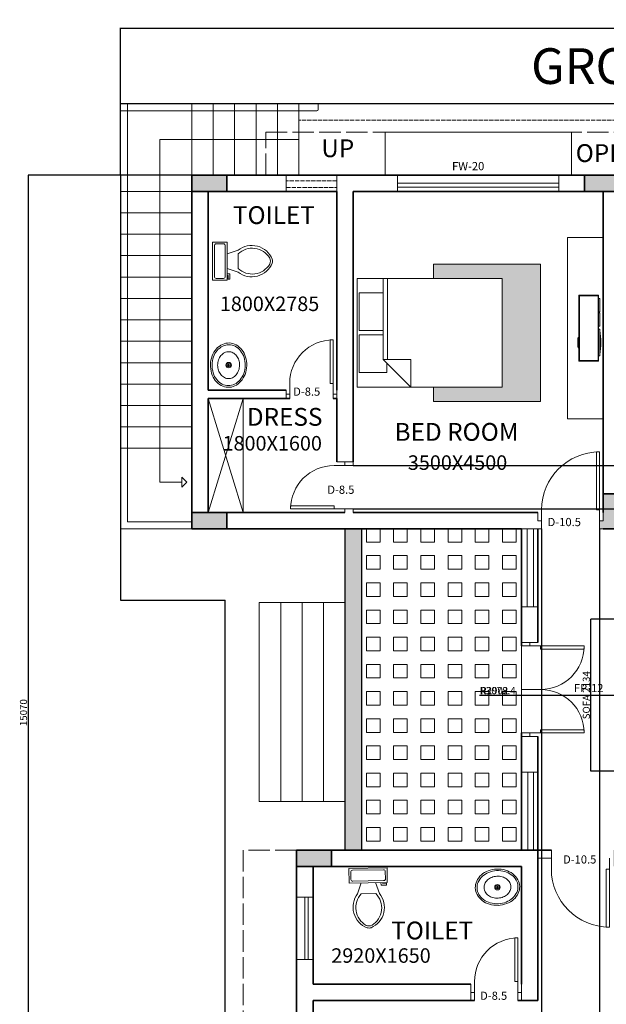
# Model space of a CAD drawing. Units: millimetres. Extents: x -17016 to 4866, y -18325 to 4338.
# Tile 2 of 5: x -17016 to -8803, y -9462 to 4338. Entities that reach past the tile are written whole.
import ezdxf

# ---------------------------------------------------------------- set-up
doc = ezdxf.new("R2010")
doc.units = ezdxf.units.MM
doc.header["$LTSCALE"] = 5
doc.linetypes.add('ACAD_ISO02W100', pattern=[15, 12, -3])
for name, color, linetype, lineweight in [('A-ANNO-DIMS', 2, 'Continuous', 18), ('A-ANNO-IDEN', 3, 'Continuous', 18), ('A-ANNO-SYMB', 7, 'Continuous', 18), ('A-ANNO-TEXT', 7, 'Continuous', 25), ('A-AREA-IDEN', 7, 'Continuous', 25), ('A-COLS', 7, 'Continuous', 35), ('A-COLS-PATT', 252, 'Continuous', 13), ('A-DOOR', 3, 'Continuous', 18), ('A-FLOR-CASE', 8, 'Continuous', 18), ('A-FLOR-FIXT', 9, 'Continuous', 18), ('A-FLOR-OTLN', 8, 'Continuous', 25), ('A-FLOR-PATT', 252, 'Continuous', 13), ('A-FLOR-STRS', 7, 'Continuous', 18), ('A-FURN', 8, 'Continuous', 18), ('A-GLAZ', 4, 'Continuous', 18), ('A-GLAZ-HIDN', 4, 'ACAD_ISO02W100', 18), ('A-ROOF', 8, 'Continuous', 18), ('A-ROOF-OVHD', 8, 'ACAD_ISO02W100', 13), ('A-WALL', 7, 'Continuous', 35)]:
    doc.layers.add(name, color=color, linetype=linetype, lineweight=lineweight)
doc.styles.get("Standard").update_dxf_attribs({"font": 'arial.ttf'})
doc.dimstyles.new('Copy of ISO-25', dxfattribs={"dimtxt": 100, "dimasz": 2.5, "dimexe": 1.25, "dimexo": 0.625, "dimtad": 1, "dimdec": 0, "dimtxsty": 'Standard', "dimcen": 2.5, "dimadec": 0, "dimazin": 0, "dimtfac": 1, "dimtdec": 0, "dimtmove": 0, "dimatfit": 3, "dimfxl": 1, "dimarcsym": 0})

# ---------------------------------------------------------------- blocks, each defined once
blk = doc.blocks.new('*U2')
for p, q in [((0, 0), (0, -6)), ((32, 0), (32, -6))]:
    blk.add_line(p, q)
blk.add_lwpolyline([(0, 0), (0, 32), (1.75, 32), (1.75, 0)], close=True)
blk.add_arc((0, 0), 32, 0, 90)
blk = doc.blocks.new('*U3')
for p, q in [((0, 0), (0, -6)), ((24, 0), (24, -6))]:
    blk.add_line(p, q)
blk.add_lwpolyline([(0, 0), (0, 24), (1.75, 24), (1.75, 0)], close=True)
blk.add_arc((0, 0), 24, 0, 90)
blk = doc.blocks.new('Bed - Queen')
for p, q in [((0, -80.00003), (0, 0)), ((0, 0), (59.99999, 0)), ((59.99999, 0), (59.99999, -80.00003)), ((7.99999, -1.2), (28.79998, -1.2)), ((7.99999, -14.4), (7.99999, -1.2)), ((28.79998, -1.2), (28.79998, -14.4)), ((31.19999, -1.2), (51.99999, -1.2)), ((31.19999, -14.4), (31.19999, -1.2)), ((51.99999, -1.2), (51.99999, -16.4)), ((0, -14.4), (44.8, -14.4)), ((59.99999, -29.6), (44.8, -14.4)), ((44.8, -14.4), (44.8, -29.6)), ((44.8, -16.8), (0, -16.8)), ((51.99999, -16.4), (46.79936, -16.4)), ((44.8, -29.6), (59.99999, -29.6)), ((59.99999, -80.00003), (0, -80.00003))]:
    blk.add_line(p, q)
blk = doc.blocks.new('Entertainment Center')
for p, q in [((-4, 0), (-5, -1)), ((4, 0), (-4, 0)), ((5, -1), (4, 0)), ((-17, -19), (-17, -1)), ((-17, -1), (43, -1)), ((-16.5, -18.5), (-16.5, -1.5)), ((-16.5, -1.5), (42.5, -1.5)), ((42.5, -1.5), (42.5, -18.5)), ((43, -1), (43, -19)), ((43, -19), (-17, -19)), ((42.5, -18.5), (-16.5, -18.5)), ((-12, -20), (-12, -19)), ((12, -20), (-12, -20)), ((12, -19), (12, -20)), ((15, -20), (15, -19)), ((27, -20), (15, -20)), ((27, -19), (27, -20)), ((28, -20), (28, -19)), ((40, -20), (28, -20)), ((40, -19), (40, -20))]:
    blk.add_line(p, q)
blk.add_arc((0, 40), 61, 259.6111, 280.3889)
blk = doc.blocks.new('*U13')
for p, q in [((9.5, -6), (9.5, -2)), ((-10, -8.5), (-8, -8.5)), ((-10, -9.5), (-10, -8.5)), ((-7, -9.5), (-10, -9.5)), ((-8, -8.5), (-8, -8)), ((-7, -8), (-7, -9.5)), ((-4, -8), (-6, -14)), ((4, -8), (6, -14)), ((4, -14), (-4, -14))]:
    blk.add_line(p, q)
blk.add_lwpolyline([(10.5, -8), (10.5, 0), (-10.5, 0), (-10.5, -8)], close=True)
for points in [[(-9.5, -2), (-9.5, -6)], [(8.5, -1), (-8.5, -1)], [(-8.5, -7), (8.5, -7)]]:
    blk.add_lwpolyline(points)
for centre, radius, start, end in [((-8.62, -1.88), 0.884, 81.8699, 188.1301), ((8.62, -1.88), 0.884, 351.8699, 98.1301), ((-8.62, -6.12), 0.884, 171.8699, 278.1301), ((8.62, -6.12), 0.884, 261.8699, 8.1301), ((3.52, -21.58), 12.17, 141.4691, 247.9714), ((4.2, -21.82), 11.33, 136.3677, 238.9468), ((-3.52, -21.58), 12.17, 292.0284, 38.5307), ((-4.2, -21.82), 11.33, 301.053, 43.6321), ((0, -27.88), 4, 245.7318, 294.2682), ((0, -29), 4, 254.8605, 285.1395)]:
    blk.add_arc(centre, radius, start, end)
blk = doc.blocks.new('Sink - Oval top')
for p, q in [((-1, 0), (1, 0)), ((0, 1), (0, -1))]:
    blk.add_line(p, q)
for points in [[(-12.23, 0.39, 0.117634), (-11.46, -3.36, 0.104469), (-8.88, -6.8, 0.090016), (-5.08, -9.07, 0.08192), (-0.32, -10.02, 0.08192), (4.49, -9.38, 0.090016), (8.42, -7.36, 0.104469), (11.22, -4.09, 0.117634), (12.23, -0.39, 0.117634), (11.46, 3.36, 0.104469), (8.88, 6.8, 0.090016), (5.08, 9.07, 0.08192), (0.32, 10.02, 0.08192), (-4.49, 9.38, 0.090016), (-8.42, 7.36, 0.104469), (-11.22, 4.09, 0.117634)], [(-11.29, 0.16, 0.118622), (-10.52, -3.25, 0.104678), (-8.07, -6.36, 0.089562), (-4.54, -8.37, 0.081185), (-0.13, -9.15, 0.081185), (4.3, -8.49, 0.089562), (7.89, -6.58, 0.104678), (10.42, -3.55, 0.118622), (11.29, -0.16, 0.118622), (10.52, 3.25, 0.104678), (8.07, 6.36, 0.089562), (4.54, 8.37, 0.081185), (0.13, 9.15, 0.081185), (-4.3, 8.49, 0.089562), (-7.89, 6.58, 0.104678), (-10.42, 3.55, 0.118622)], [(-7.42, 0.08, 0.118283), (-6.91, -2.17, 0.104607), (-5.29, -4.21, 0.089718), (-2.97, -5.53, 0.081436), (-0.07, -6.04, 0.081436), (2.84, -5.59, 0.089718), (5.2, -4.33, 0.104607), (6.86, -2.32, 0.118283), (7.42, -0.08, 0.118283), (6.91, 2.17, 0.104607), (5.29, 4.21, 0.089718), (2.97, 5.53, 0.081436), (0.07, 6.04, 0.081436), (-2.84, 5.59, 0.089718), (-5.2, 4.33, 0.104607), (-6.86, 2.32, 0.118283)]]:
    blk.add_lwpolyline(points, format="xyb", close=True)
for radius in [1.5, 1]:
    blk.add_circle((0, 0), radius)
blk = doc.blocks.new('WIN-FW20')
for p, q in [((0, 0), (0, 230)), ((2263, 0), (2263, 230)), ((0, 115), (2263, 115)), ((0, 60), (2263, 60))]:
    blk.add_line(p, q)
blk = doc.blocks.new('WIN-TOILET-875')
for p, q in [((0, 875), (230, 875)), ((115, 875), (115, 0)), ((164, 875), (164, 0)), ((0, 0), (230, 0))]:
    blk.add_line(p, q)
blk = doc.blocks.new('*D36')
at = {"layer": 'A-ANNO-DIMS', "color": 0, "lineweight": -2, "ltscale": 5, "transparency": 16777216}
for p, q in [((-8698, -4063), (-9018, -4063)), ((-9017, -6194), (-9017, -4065)), ((-8698, -6196), (-9018, -6196))]:
    blk.add_line(p, q, dxfattribs=at)
at = {"layer": 'A-ANNO-DIMS', "color": 0, "ltscale": 5, "transparency": 16777216}
for points in [[(-9017, -4065), (-9017, -4065), (-9017, -4063)], [(-9017, -6194), (-9017, -6194), (-9017, -6196)]]:
    blk.add_solid(points, dxfattribs=at)
at = {"layer": 'Defpoints', "color": 0, "ltscale": 5, "transparency": 16777216}
for p in [(-9017, -4063), (-8697, -4063), (-8697, -6196)]:
    blk.add_point(p, dxfattribs=at)
at = {"layer": 'A-ANNO-DIMS', "color": 0, "ltscale": 5, "transparency": 16777216, "insert": (-9069, -5130), "char_height": 100, "attachment_point": 5, "rotation": 90}
blk.add_mtext('SOFA 2134', dxfattribs=at)
blk = doc.blocks.new('*D46')
at = {"layer": 'A-ANNO-DIMS', "color": 0, "lineweight": -2, "ltscale": 5, "transparency": 16777216}
for p, q in [((-15606, 3162), (-15606, 4222)), ((-15604, 4221), (3521, 4221)), ((3524, 3162), (3524, 4222))]:
    blk.add_line(p, q, dxfattribs=at)
at = {"layer": 'A-ANNO-DIMS', "color": 0, "ltscale": 5, "transparency": 16777216}
for points in [[(-15604, 4221), (-15604, 4220), (-15606, 4221)], [(3521, 4221), (3521, 4220), (3524, 4221)]]:
    blk.add_solid(points, dxfattribs=at)
at = {"layer": 'Defpoints', "color": 0, "ltscale": 5, "transparency": 16777216}
for p in [(3524, 4221), (-15606, 3161), (3524, 3161)]:
    blk.add_point(p, dxfattribs=at)
at = {"layer": 'A-ANNO-DIMS', "color": 0, "ltscale": 5, "transparency": 16777216, "insert": (-6041, 4272), "char_height": 100, "attachment_point": 5}
blk.add_mtext('19130', dxfattribs=at)
blk = doc.blocks.new('*D49')
at = {"layer": 'A-ANNO-DIMS', "color": 0, "lineweight": -2, "ltscale": 5, "transparency": 16777216}
for p, q in [((-14607, 2161), (-16900, 2161)), ((-16899, 2158), (-16899, -12907)), ((-13140, -12909), (-16900, -12909))]:
    blk.add_line(p, q, dxfattribs=at)
at = {"layer": 'A-ANNO-DIMS', "color": 0, "ltscale": 5, "transparency": 16777216}
for points in [[(-16899, 2158), (-16898, 2158), (-16899, 2161)], [(-16899, -12907), (-16898, -12907), (-16899, -12909)]]:
    blk.add_solid(points, dxfattribs=at)
at = {"layer": 'Defpoints', "color": 0, "ltscale": 5, "transparency": 16777216}
for p in [(-14606, 2161), (-16899, -12909), (-13139, -12909)]:
    blk.add_point(p, dxfattribs=at)
at = {"layer": 'A-ANNO-DIMS', "color": 0, "ltscale": 5, "transparency": 16777216, "insert": (-16950, -5374), "char_height": 100, "attachment_point": 5, "rotation": 90}
blk.add_mtext('15070', dxfattribs=at)
blk = doc.blocks.new('*D50')
at = {"layer": 'A-ANNO-DIMS', "color": 0, "lineweight": -2, "ltscale": 5, "transparency": 16777216}
for p, q in [((-9709, -2800), (-9709, -18312)), ((-8896, -2800), (-8896, -18312)), ((-9707, -18311), (-8899, -18311))]:
    blk.add_line(p, q, dxfattribs=at)
at = {"layer": 'A-ANNO-DIMS', "color": 0, "ltscale": 5, "transparency": 16777216}
for points in [[(-9707, -18310), (-9707, -18311), (-9709, -18311)], [(-8899, -18310), (-8899, -18311), (-8896, -18311)]]:
    blk.add_solid(points, dxfattribs=at)
at = {"layer": 'Defpoints', "color": 0, "ltscale": 5, "transparency": 16777216}
for p in [(-9709, -2799), (-8896, -2799), (-8896, -18311)]:
    blk.add_point(p, dxfattribs=at)
at = {"layer": 'A-ANNO-DIMS', "color": 0, "ltscale": 5, "transparency": 16777216, "insert": (-9303, -18259), "char_height": 100, "attachment_point": 5}
blk.add_mtext('812.8', dxfattribs=at)
blk = doc.blocks.new('*D52')
at = {"layer": 'A-ANNO-DIMS', "color": 0, "lineweight": -2, "ltscale": 5, "transparency": 16777216}
for p, q in [((-12346, -1910), (4853, -1910)), ((4852, -2517), (4852, -1912)), ((-12346, -2519), (4853, -2519))]:
    blk.add_line(p, q, dxfattribs=at)
at = {"layer": 'A-ANNO-DIMS', "color": 0, "ltscale": 5, "transparency": 16777216}
for points in [[(4851, -1912), (4852, -1912), (4852, -1910)], [(4851, -2517), (4852, -2517), (4852, -2519)]]:
    blk.add_solid(points, dxfattribs=at)
at = {"layer": 'Defpoints', "color": 0, "ltscale": 5, "transparency": 16777216}
for p in [(-12346, -1910), (4852, -1910), (-12346, -2519)]:
    blk.add_point(p, dxfattribs=at)
at = {"layer": 'A-ANNO-DIMS', "color": 0, "ltscale": 5, "transparency": 16777216, "insert": (4800, -2214), "char_height": 100, "attachment_point": 5, "rotation": 90}
blk.add_mtext('609.6', dxfattribs=at)
blk = doc.blocks.new('*D57')
at = {"layer": 'A-ANNO-DIMS', "color": 0, "lineweight": -2, "ltscale": 5, "transparency": 16777216}
for p, q in [((-10580, -5130), (-8479, -5130)), ((-5398, -5130), (-8477, -5130))]:
    blk.add_line(p, q, dxfattribs=at)
at = {"layer": 'A-ANNO-DIMS', "color": 0, "ltscale": 5, "transparency": 16777216}
blk.add_solid([(-8479, -5129), (-8479, -5130), (-8477, -5130)], dxfattribs=at)
at = {"layer": 'Defpoints', "color": 0, "ltscale": 5, "transparency": 16777216}
for p in [(-8477, -5130), (-5398, -5130)]:
    blk.add_point(p, dxfattribs=at)
at = {"layer": 'A-ANNO-DIMS', "color": 0, "ltscale": 5, "transparency": 16777216, "insert": (-10324, -5078), "char_height": 100, "attachment_point": 5}
blk.add_mtext('R3078.4', dxfattribs=at)
blk = doc.blocks.new('*D58')
at = {"layer": 'A-ANNO-DIMS', "color": 0, "lineweight": -2, "ltscale": 5, "transparency": 16777216}
for p, q in [((-10568, -5130), (-8632, -5130)), ((-5727, -5130), (-8629, -5130))]:
    blk.add_line(p, q, dxfattribs=at)
at = {"layer": 'A-ANNO-DIMS', "color": 0, "ltscale": 5, "transparency": 16777216}
blk.add_solid([(-8632, -5129), (-8632, -5130), (-8629, -5130)], dxfattribs=at)
at = {"layer": 'Defpoints', "color": 0, "ltscale": 5, "transparency": 16777216}
for p in [(-8629, -5130), (-5727, -5130)]:
    blk.add_point(p, dxfattribs=at)
at = {"layer": 'A-ANNO-DIMS', "color": 0, "ltscale": 5, "transparency": 16777216, "insert": (-10370, -5078), "char_height": 100, "attachment_point": 5}
blk.add_mtext('R2902', dxfattribs=at)

msp = doc.modelspace()

# ---------------------------------------------------------------- hatches: boundary and pattern name
at = {"layer": 'A-COLS-PATT', "ltscale": 5}
h = msp.add_hatch(color=256, dxfattribs=at)
h.dxf.hatch_style = 1
h.paths.add_polyline_path([(2523.62, 2160.89), (2293.62, 2160.89), (2293.62, 1930.89), (2293.62, 1670.89), (2523.62, 1670.89)])
h.paths.add_polyline_path([(-14116.35, 2160.89), (-14606.38, 2160.89), (-14606.38, 1930.89), (-14116.35, 1930.89)])
h = msp.add_hatch(color=256, dxfattribs=at)
h.dxf.hatch_style = 1
h.paths.add_polyline_path([(-8616.38, 2160.89), (-9107.57, 2160.89), (-9107.57, 1930.89), (-8846.38, 1930.89), (-8616.38, 1930.89)])
h = msp.add_hatch(color=256, dxfattribs=at)
h.dxf.hatch_style = 1
h.paths.add_polyline_path([(2523.62, -2569.11), (2033.62, -2569.11), (2033.62, -2799.11), (2523.62, -2799.11)])
h.paths.add_polyline_path([(-1909.18, -2569.11), (-2399.18, -2569.11), (-2399.18, -2799.11), (-1909.18, -2799.11)])
h.paths.add_polyline_path([(-5436.38, -2309.11), (-5666.38, -2309.11), (-5666.38, -2569.11), (-5666.38, -2684.11), (-5716.38, -2684.11), (-5716.38, -2799.11), (-5436.38, -2799.11)])
h.paths.add_polyline_path([(-8616.38, -2309.11), (-8846.38, -2309.11), (-8846.38, -2569.11), (-8846.38, -2684.11), (-8896.38, -2684.11), (-8896.38, -2799.11), (-8846.38, -2799.11), (-8616.38, -2799.11)])
h = msp.add_hatch(color=256, dxfattribs=at)
h.dxf.hatch_style = 1
h.paths.add_polyline_path([(-14116.38, -2569.11), (-14606.38, -2569.11), (-14606.38, -2799.11), (-14116.38, -2799.11)])
h = msp.add_hatch(color=256, dxfattribs=at)
h.dxf.hatch_style = 1
h.paths.add_polyline_path([(980.82, -7299.11), (490.82, -7299.11), (490.82, -7529.11), (980.82, -7529.11)])
h.paths.add_polyline_path([(-3449.18, -7414.11), (-3399.18, -7414.11), (-3399.18, -7299.11), (-3939.18, -7299.11), (-3939.18, -7529.11), (-3449.18, -7529.11)])
h.paths.add_polyline_path([(-8219.18, -7299.11), (-8709.18, -7299.11), (-8709.18, -7529.11), (-8219.18, -7529.11)])
h.paths.add_polyline_path([(-12649.22, -7299.11), (-13139.18, -7299.11), (-13139.18, -7529.11), (-12649.22, -7529.11)])
at = {"layer": 'A-FLOR-PATT'}
h = msp.add_hatch(dxfattribs=at)
h.set_pattern_fill('ANSI38', color=256, scale=25)
h.set_pattern_definition([(45, (-20162.07, -7174.37), (-56.1266, 56.1266), []), (135, (-20162.07, -7174.37), (-168.3798, 56.1266), [198.4375, -119.0625])])
h.paths.add_polyline_path([(-1358.58, -10190.51), (-396.23, -10190.51), (-396.23, -9990.51), (-1896.23, -9990.51), (-1896.23, -11914.51), (-396.23, -11914.51), (-396.23, -11714.51), (-1358.58, -11714.51)])
h.paths.add_polyline_path([(-10262.12, -9990.51), (-11762.12, -9990.51), (-11762.12, -10190.51), (-10799.77, -10190.51), (-10799.77, -11714.51), (-11762.12, -11714.51), (-11762.12, -11914.51), (-10262.12, -11914.51)])
h.paths.add_polyline_path([(-9722.08, 912.47), (-11222.08, 912.47), (-11222.08, 712.47), (-10260.08, 712.47), (-10260.08, -811.53), (-11222.08, -811.53), (-11222.08, -1011.53), (-9722.08, -1011.53)])
h.paths.add_polyline_path([(-2814.18, 912.47), (-4314.18, 912.47), (-4314.18, 712.47), (-3352.18, 712.47), (-3352.18, -811.53), (-4314.18, -811.53), (-4314.18, -1011.53), (-2814.18, -1011.53)])
h = msp.add_hatch(dxfattribs=at)
h.set_pattern_fill('ANGLE', color=256, scale=25)
h.set_pattern_definition([(0, (-20162.07, -7174.37), (0, 174.625), [127, -47.625]), (90, (-20162.07, -7174.37), (-174.625, 1e-14), [127, -47.625])])
h.paths.add_polyline_path([(72.82, -2799.11), (-157.18, -2799.11), (-157.18, -7299.11), (72.82, -7299.11)])
h.paths.add_polyline_path([(-12231.38, -2799.11), (-12461.38, -2799.11), (-12461.38, -7299.11), (-12231.38, -7299.11)])
h = msp.add_hatch(dxfattribs=at)
h.set_pattern_fill('SQUARE', color=256, scale=60)
h.set_pattern_definition([(0, (-20162.07, -7174.37), (0, 190.5), [190.5, -190.5]), (90, (-20162.07, -7174.37), (-190.5, 1e-14), [190.5, -190.5])])
h.paths.add_polyline_path([(-157.18, -2799.11), (-436.38, -2799.11), (-2169.18, -2799.11), (-2169.18, -4439.51), (-2169.18, -5658.71), (-2169.18, -7299.11), (-157.18, -7299.11)])
h.paths.add_polyline_path([(-9989.18, -4439.51), (-9989.18, -2799.11), (-12231.38, -2799.11), (-12231.38, -7299.11), (-9989.18, -7299.11), (-9989.18, -5658.71)])

# ---------------------------------------------------------------- linework, layer by layer
at = {"layer": 'A-ANNO-SYMB', "ltscale": 5}
for p, q in [((-13106.38, 2660.89), (-15056.38, 2660.89)), ((-15056.38, -2144.06), (-15056.38, 2660.89)), ((-15056.38, -2144.06), (-14746.23, -2144.06)), ((-14677.51, -2144.06), (-14747.98, -2072.05)), ((-14744.58, -2211.6), (-14747.98, -2072.05)), ((-14677.51, -2144.06), (-14744.58, -2211.6))]:
    msp.add_line(p, q, dxfattribs=at)
at = {"layer": 'A-COLS', "ltscale": 5}
for p, q in [((-14116.35, 1930.89), (-14116.35, 2160.89)), ((-9107.57, 1930.89), (-9107.57, 2160.89)), ((-8846.38, 1930.89), (-8616.38, 1930.89)), ((-8616.38, -2309.11), (-8846.38, -2309.11)), ((-14116.38, -2569.11), (-14116.38, -2799.11)), ((-12649.22, -7529.11), (-12649.22, -7299.11))]:
    msp.add_line(p, q, dxfattribs=at)
at = {"layer": 'A-DOOR'}
for p, q in [((-13285.98, -911.61), (-13285.98, -854.11)), ((-13285.98, -900.76), (-13285.98, -969.11)), ((-13235.98, -911.61), (-13285.98, -911.61)), ((-13235.98, -911.61), (-13235.98, -969.11)), ((-12626.38, -911.61), (-12626.38, -854.11)), ((-12576.38, -911.61), (-12626.38, -911.61)), ((-12626.38, -911.61), (-12626.38, -969.11)), ((-12576.38, -854.11), (-12576.38, -969.11)), ((-12461.38, -1859.51), (-12576.38, -1859.51)), ((-12461.38, -1909.51), (-12461.38, -1859.51)), ((-12461.38, -1859.51), (-12346.38, -1859.51)), ((-12461.38, -1909.51), (-12346.38, -1909.51)), ((-12346.38, -1859.51), (-12346.38, -1909.51)), ((-12461.38, -2519.11), (-12576.38, -2519.11)), ((-12461.38, -2569.11), (-12461.38, -2519.11)), ((-12461.38, -2519.11), (-12346.38, -2519.11)), ((-12346.38, -2519.11), (-12346.38, -2569.11)), ((-9759.18, -2684.11), (-9759.18, -2569.11)), ((-8846.38, -2569.11), (-8846.38, -2684.11)), ((-9709.18, -2684.11), (-9759.18, -2684.11)), ((-9709.18, -2684.11), (-9709.18, -2799.11)), ((-8846.38, -2684.11), (-8896.38, -2684.11)), ((-8896.38, -2684.11), (-8896.38, -2799.11)), ((-9759.18, -2799.11), (-9709.18, -2799.11)), ((-8846.38, -2799.11), (-8896.38, -2799.11)), ((-9874.18, -4389.51), (-9989.18, -4389.51)), ((-9874.18, -4439.51), (-9874.18, -4389.51)), ((-9874.18, -4389.51), (-9759.18, -4389.51)), ((-9874.18, -4439.51), (-9989.18, -4439.51)), ((-9989.18, -4439.51), (-9989.18, -5658.71)), ((-9759.18, -5049.11), (-9989.18, -5049.11)), ((-9874.18, -5658.71), (-9989.18, -5658.71)), ((-9874.18, -5708.71), (-9989.18, -5708.71)), ((-9874.18, -5658.71), (-9874.18, -5708.71)), ((-9874.18, -5708.71), (-9759.18, -5708.71)), ((-9571.98, -7414.11), (-9571.98, -7299.11)), ((-9571.98, -7414.11), (-9759.18, -7413.87)), ((-10698.76, -9295.33), (-10698.76, -9179.11)), ((-10039.18, -9294.11), (-10039.18, -9179.11)), ((-9989.18, -9179.11), (-9989.18, -9409.11)), ((-10648.78, -9294.11), (-10698.76, -9295.33)), ((-10698.76, -9295.33), (-10698.76, -9409.11)), ((-10648.78, -9294.11), (-10648.78, -9409.11)), ((-9989.18, -9294.11), (-10039.18, -9294.11)), ((-10039.18, -9294.11), (-10039.18, -9409.11))]:
    msp.add_line(p, q, dxfattribs=at)
at = {"layer": 'A-FLOR-CASE'}
for p, q in [((-13888.29, -2569.11), (-14376.38, -969.11)), ((-14376.38, -2569.11), (-13888.29, -969.11)), ((-13888.29, -969.11), (-13888.29, -2569.11))]:
    msp.add_line(p, q, dxfattribs=at)
at = {"layer": 'A-FLOR-OTLN', "ltscale": 5}
for p, q in [((-15606.38, 2160.89), (-15606.38, 3160.89)), ((-14606.38, 3160.89), (-15606.38, 3160.89)), ((-15606.38, 2160.89), (-15606.38, -2799.11)), ((-15606.38, -2799.11), (-15606.38, -3799.11)), ((-15606.38, -3799.11), (-14653.77, -3799.11)), ((-14653.77, -3799.11), (-14139.18, -3799.11)), ((-14139.18, -13909.11), (-14139.18, -3799.11))]:
    msp.add_line(p, q, dxfattribs=at)
at = {"layer": 'A-FLOR-OTLN'}
for p, q in [((2523.62, 3160.89), (-14606.38, 3160.89)), ((-12461.38, -2799.11), (-12461.38, -7299.11)), ((-12231.38, -2799.11), (-12231.38, -7299.11))]:
    msp.add_line(p, q, dxfattribs=at)
at = {"layer": 'A-FLOR-PATT'}
msp.add_lwpolyline([(-11222.08, -811.53), (-11222.08, -1011.53), (-9722.08, -1011.53), (-9722.08, 912.47), (-11222.08, 912.47), (-11222.08, 712.47)], dxfattribs=at)
at = {"layer": 'A-FLOR-STRS', "ltscale": 5}
for p, q in [((-14606.38, 3060.89), (-15606.38, 3060.89)), ((-15506.38, 2160.89), (-15506.38, 3160.89)), ((-14606.38, 2160.89), (-14606.38, 3160.89)), ((-14306.38, 2160.89), (-14306.38, 3160.89)), ((-14006.38, 2160.89), (-14006.38, 3160.89)), ((-13706.38, 2160.89), (-13706.38, 3160.89)), ((-13406.38, 2160.89), (-13406.38, 3160.89)), ((-13106.38, 2160.89), (-13106.38, 3160.89)), ((-12835.49, 3080.89), (-12835.49, 3160.89)), ((-15506.38, 2160.89), (-15506.38, -2699.11)), ((-14606.38, 1930.89), (-15606.38, 1930.89)), ((-14606.38, 1630.89), (-15606.38, 1630.89)), ((-14606.38, 1330.89), (-15606.38, 1330.89)), ((-14606.38, 1030.89), (-15606.38, 1030.89)), ((-14606.38, 730.89), (-15606.38, 730.89)), ((-14606.38, 430.89), (-15606.38, 430.89)), ((-14606.38, 130.89), (-15606.38, 130.89)), ((-14606.38, -169.11), (-15606.38, -169.11)), ((-14606.38, -469.11), (-15606.38, -469.11)), ((-14606.38, -769.11), (-15606.38, -769.11)), ((-14606.38, -1069.11), (-15606.38, -1069.11)), ((-14606.38, -1369.11), (-15606.38, -1369.11)), ((-14606.38, -1669.11), (-15606.38, -1669.11)), ((-14606.38, -2699.11), (-15506.38, -2699.11)), ((-14606.38, -2799.11), (-15606.38, -2799.11)), ((-13661.38, -3831.79), (-13661.38, -6618.73)), ((-12461.38, -3831.79), (-13661.38, -3831.79)), ((-13361.38, -3831.79), (-13361.38, -6618.73)), ((-13061.38, -3831.79), (-13061.38, -6618.73)), ((-12761.38, -3831.79), (-12761.38, -6618.73)), ((-12461.38, -6618.73), (-13661.38, -6618.73))]:
    msp.add_line(p, q, dxfattribs=at)
at = {"layer": 'A-FLOR-STRS'}
msp.add_line((-12855.49, 3060.89), (-14606.38, 3060.89), dxfattribs=at)
msp.add_arc((-12855.49, 3080.89), 20, 270, 0, dxfattribs=at)
at = {"layer": 'A-FURN'}
msp.add_line((-10260.08, 712.47), (-11222.08, 712.47), dxfattribs=at)
msp.add_lwpolyline([(-8846.38, -1258.32), (-9346.38, -1258.32), (-9346.38, 1287.26), (-8846.38, 1287.26)], dxfattribs=at)
at = {"layer": 'A-GLAZ'}
for p, q in [((-13282.97, 1930.89), (-13282.97, 2160.89)), ((-12576.38, 1930.89), (-12576.38, 2160.89)), ((-9989.18, -2799.11), (-9759.18, -2799.11)), ((-9908.8, -3889.51), (-9908.8, -2799.11)), ((-9820.98, -3889.51), (-9820.98, -2799.11)), ((-9759.18, -3889.51), (-9989.18, -3889.51)), ((-9759.18, -6208.71), (-9989.18, -6208.71)), ((-9903.32, -7299.11), (-9903.32, -6208.71)), ((-9823.63, -6208.71), (-9823.63, -7299.11))]:
    msp.add_line(p, q, dxfattribs=at)
at = {"layer": 'A-GLAZ-HIDN'}
for p, q in [((-12576.38, 2081.77), (-13282.97, 2081.77)), ((-13282.97, 1985.53), (-12576.38, 1985.53))]:
    msp.add_line(p, q, dxfattribs=at)
at = {"layer": 'A-ROOF', "ltscale": 5}
for p, q in [((-11901.19, 2160.89), (-11901.19, 2760.89)), ((-11901.19, 2760.89), (-9169.02, 2760.89)), ((-9290.77, 2160.89), (-9290.77, 2760.89))]:
    msp.add_line(p, q, dxfattribs=at)
at = {"layer": 'A-ROOF-OVHD'}
msp.add_line((2293.62, 2930.89), (-13106.38, 2930.89), dxfattribs=at)
at = {"layer": 'A-ROOF-OVHD', "ltscale": 5}
for p, q in [((-13570.85, 2160.89), (-13570.85, 2760.89)), ((-13570.85, 2760.89), (874.92, 2760.89)), ((-13139.18, -7299.11), (-13889.18, -7299.11)), ((-13889.18, -7299.11), (-13889.18, -13655.43))]:
    msp.add_line(p, q, dxfattribs=at)
at = {"layer": 'A-WALL'}
for p, q in [((2523.62, 2160.89), (-14606.38, 2160.89)), ((-14606.38, 2160.89), (-14606.38, -2799.11)), ((-12576.38, 1930.89), (-14606.38, 1930.89)), ((-14376.38, 1930.89), (-14376.38, -854.11)), ((-12576.38, 1930.89), (-12576.38, -854.11)), ((-12346.38, 1930.89), (-12346.38, -1859.51)), ((-8846.38, 1930.89), (-12346.38, 1930.89)), ((-8846.38, 1930.89), (-8846.38, -2569.11)), ((-13285.98, -854.11), (-14376.38, -854.11)), ((-14376.38, -969.11), (-14376.38, -2569.11)), ((-13235.98, -969.11), (-14376.38, -969.11)), ((-12576.38, -969.11), (-12626.38, -969.11)), ((-12576.38, -969.11), (-12576.38, -1859.51)), ((-12576.38, -2569.11), (-14606.38, -2569.11)), ((-12576.38, -2569.11), (-12461.38, -2569.11)), ((-9759.18, -2569.11), (-12346.38, -2569.11)), ((-9989.18, -2799.11), (-14606.38, -2799.11)), ((-9989.18, -2799.11), (-9989.18, -4439.51)), ((-9759.18, -2799.11), (-9759.18, -4389.51)), ((-6477.58, -2799.11), (-8846.38, -2799.11)), ((-9989.18, -5658.71), (-9989.18, -7299.11)), ((-9759.18, -5708.71), (-9759.18, -7413.87)), ((-12461.38, -7299.11), (-13139.18, -7299.11)), ((-13139.18, -7529.11), (-13139.18, -7299.11)), ((-9571.98, -7299.11), (-12461.38, -7299.11)), ((-9759.18, -7413.87), (-9759.18, -9409.11)), ((-13139.18, -7529.11), (-13139.18, -12909.11)), ((-9989.18, -7529.11), (-13139.18, -7529.11)), ((-12909.18, -7529.11), (-12909.18, -9179.11)), ((-9989.18, -7529.11), (-9989.18, -9179.11)), ((-10698.76, -9179.11), (-12909.18, -9179.11)), ((-12909.18, -9409.11), (-12909.18, -12909.11)), ((-10648.78, -9409.11), (-12909.18, -9409.11)), ((-9759.18, -9409.11), (-10039.18, -9409.11))]:
    msp.add_line(p, q, dxfattribs=at)

# ---------------------------------------------------------------- block references
at = {"layer": 'A-DOOR', "xscale": -25.4, "yscale": 25.4, "zscale": 25.4}
for name, p in [('*U3', (-12626.38, -759.21)), ('*U2', (-8896.38, -2531.71)), ('*U3', (-10039.18, -9141.71))]:
    msp.add_blockref(name, p, dxfattribs=at)
at = {"layer": 'A-DOOR', "yscale": 25.4, "zscale": 25.4}
for name, p, xscale, rotation in [('*U3', (-12613.78, -2519.11), 25.4, 90.00000000000003), ('*U3', (-9721.78, -4439.51), 25.4, 270), ('*U3', (-9721.78, -5658.71), -25.4, 270), ('*U2', (-8759.18, -7566.51), 25.4, 180)]:
    msp.add_blockref(name, p, dxfattribs=dict(at, xscale=xscale, rotation=rotation))
at = {"layer": 'A-FLOR-FIXT', "yscale": 25.4, "zscale": 25.4}
for name, p, xscale, rotation in [('*U13', (-14315.06, 954.14), 25.4, 90), ('Sink - Oval top', (-14090.93, -503.77), 25.4, 90), ('*U13', (-12139.29, -7554.18), -25.4, 1.060997950081761), ('Sink - Oval top', (-10326.18, -7820.12), 25.4, 3.833934461057109)]:
    msp.add_blockref(name, p, dxfattribs=dict(at, xscale=xscale, rotation=rotation))
at = {"layer": 'A-FURN', "extrusion": (-1e-16, 0, -1), "xscale": 25.4, "yscale": 25.4, "zscale": 25.4, "rotation": 269.9999999999998}
msp.add_blockref('Bed - Queen', (12292.09, 712.47), dxfattribs=at)
at = {"layer": 'A-FURN', "xscale": 15.40069445834287, "yscale": 15.40069445834287, "zscale": 15.40069445834287, "rotation": 89.99999999999999}
msp.add_blockref('Entertainment Center', (-9202.41, -186.34), dxfattribs=at)
at = {"layer": 'A-GLAZ'}
for name, p in [('WIN-FW20', (-11727.99, 1930.89)), ('WIN-TOILET-875', (-13139.18, -8833.76))]:
    msp.add_blockref(name, p, dxfattribs=at)

# ---------------------------------------------------------------- texts
at = {"layer": 'A-ANNO-IDEN', "ltscale": 5}
for s, p in [('FW-20', (-10963.02, 2227.86)), ('D-8.5', (-13187.27, -932.1)), ('D-8.5', (-12709.04, -2307.04)), ('D-10.5', (-9624.35, -2759.93)), ('FP-12', (-9256.42, -5086.86)), ('D-10.5', (-9408.23, -7488.78)), ('D-8.5', (-10569.88, -9398.89))]:
    msp.add_text(s, height=114.837, dxfattribs=at).set_placement(p)
at = {"layer": 'A-ANNO-TEXT', "ltscale": 5}
for s, height, p in [('GROUND FLOOR PLAN', 500, (-9855.74, 3437.79)), ('UP', 250, (-12793.71, 2410.98))]:
    msp.add_text(s, height=height, dxfattribs=at).set_placement(p)
at = {"layer": 'A-AREA-IDEN', "ltscale": 5}
for s, height, p in [('OPEN PLATFORM 1000 WIDE', 250, (-9230.64, 2343.25)), ('TOILET', 250, (-14030.31, 1474.11)), ('1800X2785', 203.546, (-14213.82, 254.48)), ('DRESS', 250, (-13835.7, -1353.53)), ('BED ROOM', 250, (-11766.96, -1564.16)), ('1800X1600', 203.546, (-14176.38, -1700.5)), ('3500X4500', 203.546, (-11581.53, -1971.29)), ('TOILET', 250, (-11814.45, -8552.29)), ('2920X1650', 203.546, (-12653.45, -8880.03))]:
    msp.add_text(s, height=height, dxfattribs=at).set_placement(p)

# ---------------------------------------------------------------- dimensions: what is measured, and where the dimension line sits
at = {"layer": 'A-ANNO-DIMS', "ltscale": 5}
for base, p1, p2, override, picture, middle in [((3523.62, 4220.64), (-15606.38, 3160.89), (3523.62, 3160.89), {"dimdec": 0, "dimlfac": 1, "dimrnd": 0, "dimzin": 0, "dimdsep": 46, "dimlunit": 2}, '*D46', (-6041.38, 4272.35)), ((-8896.38, -18310.58), (-9709.18, -2799.11), (-8896.38, -2799.11), {"dimdec": 1, "dimlfac": 1, "dimrnd": 0, "dimzin": 0, "dimdsep": 46, "dimlunit": 2}, '*D50', (-9302.78, -18258.9))]:
    dim = msp.add_linear_dim(base=base, p1=p1, p2=p2, dimstyle='Copy of ISO-25', override=override, dxfattribs=at)
    dim.commit()
    dim.dimension.update_dxf_attribs({"geometry": picture, "text_midpoint": middle})
for base, p1, p2, override, picture, middle in [((-16898.81, -12909.11), (-14606.38, 2160.89), (-13139.18, -12909.11), {"dimdec": 0, "dimlfac": 1, "dimrnd": 0, "dimzin": 0, "dimdsep": 46, "dimlunit": 2}, '*D49', (-16950.49, -5374.11)), ((4851.91, -1909.51), (-12346.38, -2519.11), (-12346.38, -1909.51), {"dimdec": 1, "dimlfac": 1, "dimrnd": 0, "dimzin": 0, "dimdsep": 46, "dimlunit": 2}, '*D52', (4800.22, -2214.31))]:
    dim = msp.add_linear_dim(base=base, p1=p1, p2=p2, angle=90, dimstyle='Copy of ISO-25', override=override, dxfattribs=at)
    dim.commit()
    dim.dimension.update_dxf_attribs({"geometry": picture, "text_midpoint": middle})
dim = msp.add_linear_dim(base=(-9016.98, -4062.86), p1=(-8696.94, -6196.46), p2=(-8696.94, -4062.86), angle=89.999979, text='SOFA <>', dimstyle='Copy of ISO-25', override={"dimdec": 0, "dimlfac": 1, "dimrnd": 0, "dimzin": 0, "dimdsep": 46, "dimlunit": 2}, dxfattribs=at)
dim.commit()
dim.dimension.update_dxf_attribs({"geometry": '*D36', "text_midpoint": (-9069.38, -5129.66)})
for center, mpoint, override, picture, middle in [((-5398.41, -5129.66), (-8476.81, -5129.66), {"dimdec": 1, "dimlfac": 1, "dimrnd": 0, "dimzin": 0, "dimdsep": 46, "dimlunit": 2}, '*D57', (-10323.85, -5129.66)), ((-5727.26, -5129.66), (-8629.21, -5129.66), {"dimdec": 0, "dimlfac": 1, "dimrnd": 0, "dimzin": 0, "dimdsep": 46, "dimlunit": 2}, '*D58', (-10370.38, -5129.66))]:
    dim = msp.add_radius_dim(center=center, mpoint=mpoint, dimstyle='Copy of ISO-25', override=override, dxfattribs=at)
    dim.commit()
    dim.dimension.update_dxf_attribs({"geometry": picture, "text_midpoint": middle, "dimtype": 164})

doc.saveas('drawing.dxf')
